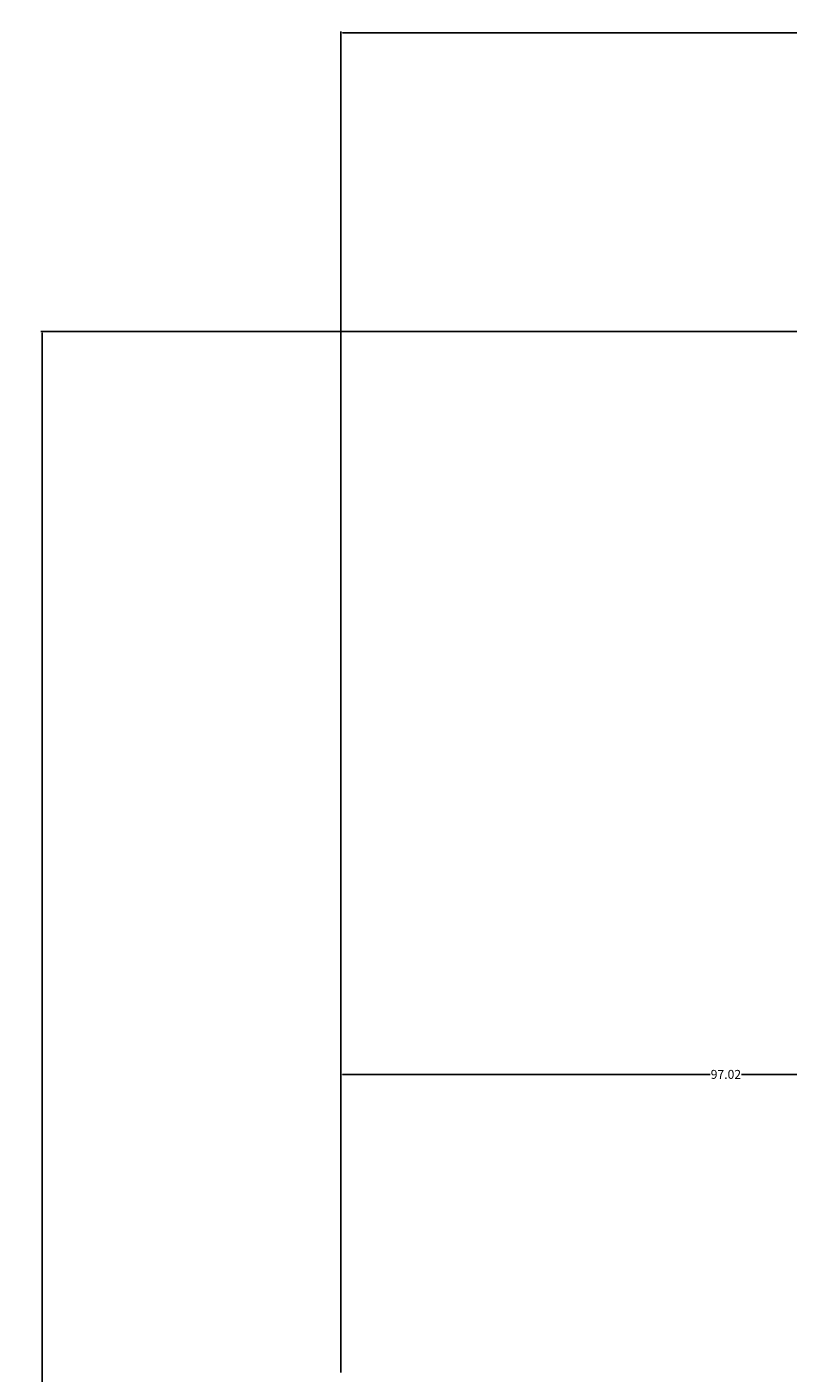
# Model space of a CAD drawing. Units: inches. Extents: x 8 to 634, y 41 to 867.
# Tile 16 of 21: x 8 to 104, y 698 to 867. Entities that reach past the tile are written whole.
import ezdxf

# ---------------------------------------------------------------- set-up
doc = ezdxf.new("R2010")
doc.units = ezdxf.units.IN
doc.header["$MEASUREMENT"] = 0
doc.layers.add('A-ANNO-DIMS', color=2, linetype='Continuous', lineweight=18)
doc.styles.get("Standard").update_dxf_attribs({"font": 'arial.ttf'})
doc.dimstyles.get("Standard").update_dxf_attribs({"dimtxt": 1.125, "dimasz": 0.18, "dimexe": 0.18, "dimexo": 0.0625, "dimgap": 0.09, "dimtad": 0, "dimtih": 1, "dimtoh": 1, "dimdec": 4, "dimzin": 0, "dimdsep": 46, "dimlunit": 4, "dimtxsty": 'Standard', "dimcen": 0.09, "dimadec": 0, "dimazin": 0, "dimtfac": 1, "dimtdec": 4, "dimtofl": 0, "dimtmove": 0, "dimatfit": 3, "dimfxl": 1, "dimtolj": 1, "dimtzin": 0, "dimarcsym": 0})

# ---------------------------------------------------------------- blocks, each defined once
blk = doc.blocks.new('*D19')
at = {"layer": 'A-ANNO-DIMS', "color": 0, "lineweight": -2, "transparency": 16777216}
for p, q in [((47.34, 697.73), (47.34, 866.81)), ((47.52, 866.63), (319.51, 866.63)), ((594.17, 866.63), (322.18, 866.63)), ((594.35, 827.83), (594.35, 866.81))]:
    blk.add_line(p, q, dxfattribs=at)
at = {"layer": 'A-ANNO-DIMS', "color": 0, "transparency": 16777216}
for points in [[(47.52, 866.66), (47.52, 866.6), (47.34, 866.63)], [(594.17, 866.66), (594.17, 866.6), (594.35, 866.63)]]:
    blk.add_solid(points, dxfattribs=at)
at = {"layer": 'Defpoints', "color": 0, "transparency": 16777216}
for p in [(594.35, 866.63), (594.35, 827.77), (47.34, 697.67)]:
    blk.add_point(p, dxfattribs=at)
at = {"layer": 'A-ANNO-DIMS', "color": 0, "transparency": 16777216, "insert": (320.85, 866.63), "char_height": 1.125, "attachment_point": 5}
blk.add_mtext('\\A1;547', dxfattribs=at)
blk = doc.blocks.new('*D20')
at = {"layer": 'A-ANNO-DIMS', "color": 0, "lineweight": -2, "transparency": 16777216}
for p, q in [((144.29, 828.98), (9.51, 828.98)), ((9.69, 828.8), (9.69, 454.93)), ((9.69, 79.74), (9.69, 453.6)), ((47.28, 79.56), (9.51, 79.56))]:
    blk.add_line(p, q, dxfattribs=at)
at = {"layer": 'A-ANNO-DIMS', "color": 0, "transparency": 16777216}
for points in [[(9.66, 828.8), (9.72, 828.8), (9.69, 828.98)], [(9.66, 79.74), (9.72, 79.74), (9.69, 79.56)]]:
    blk.add_solid(points, dxfattribs=at)
at = {"layer": 'Defpoints', "color": 0, "transparency": 16777216}
for p in [(9.69, 828.98), (144.36, 828.98), (47.34, 79.56)]:
    blk.add_point(p, dxfattribs=at)
at = {"layer": 'A-ANNO-DIMS', "color": 0, "transparency": 16777216, "insert": (9.69, 454.27), "char_height": 1.125, "attachment_point": 5}
blk.add_mtext('\\A1;749.4', dxfattribs=at)
blk = doc.blocks.new('*D22')
at = {"layer": 'A-ANNO-DIMS', "color": 0, "lineweight": -2, "transparency": 16777216}
for p, q in [((47.34, 697.73), (47.34, 735.5)), ((47.52, 735.32), (93.87, 735.32)), ((144.18, 735.32), (97.83, 735.32)), ((144.36, 697.73), (144.36, 735.5))]:
    blk.add_line(p, q, dxfattribs=at)
at = {"layer": 'A-ANNO-DIMS', "color": 0, "transparency": 16777216}
for points in [[(47.52, 735.35), (47.52, 735.29), (47.34, 735.32)], [(144.18, 735.35), (144.18, 735.29), (144.36, 735.32)]]:
    blk.add_solid(points, dxfattribs=at)
at = {"layer": 'Defpoints', "color": 0, "transparency": 16777216}
for p in [(144.36, 735.32), (47.34, 697.67), (144.36, 697.67)]:
    blk.add_point(p, dxfattribs=at)
at = {"layer": 'A-ANNO-DIMS', "color": 0, "transparency": 16777216, "insert": (95.85, 735.32), "char_height": 1.125, "attachment_point": 5}
blk.add_mtext('\\A1;97.02', dxfattribs=at)

msp = doc.modelspace()

# ---------------------------------------------------------------- dimensions: what is measured, and where the dimension line sits
at = {"layer": 'A-ANNO-DIMS'}
for base, p2, override, picture, middle in [((594.3501, 866.6321), (594.3501, 827.7671), {"dimdec": 0, "dimlfac": 1, "dimrnd": 0, "dimzin": 0, "dimdsep": 46, "dimlunit": 2}, '*D19', (320.8451, 866.6321)), ((144.3564, 735.3155), (144.3564, 697.6655), {"dimdec": 2, "dimlfac": 1, "dimrnd": 0, "dimzin": 0, "dimdsep": 46, "dimlunit": 2}, '*D22', (95.8482, 735.3155))]:
    dim = msp.add_linear_dim(base=base, p1=(47.3401, 697.6655), p2=p2, dimstyle='Standard', override=override, dxfattribs=at)
    dim.commit()
    dim.dimension.update_dxf_attribs({"geometry": picture, "text_midpoint": middle})
dim = msp.add_linear_dim(base=(9.6901, 828.9821), p1=(47.3401, 79.5555), p2=(144.3564, 828.9821), angle=90, dimstyle='Standard', override={"dimdec": 1, "dimlfac": 1, "dimrnd": 0, "dimzin": 0, "dimdsep": 46, "dimlunit": 2}, dxfattribs=at)
dim.commit()
dim.dimension.update_dxf_attribs({"geometry": '*D20', "text_midpoint": (9.6901, 454.2688)})

doc.saveas('drawing.dxf')
